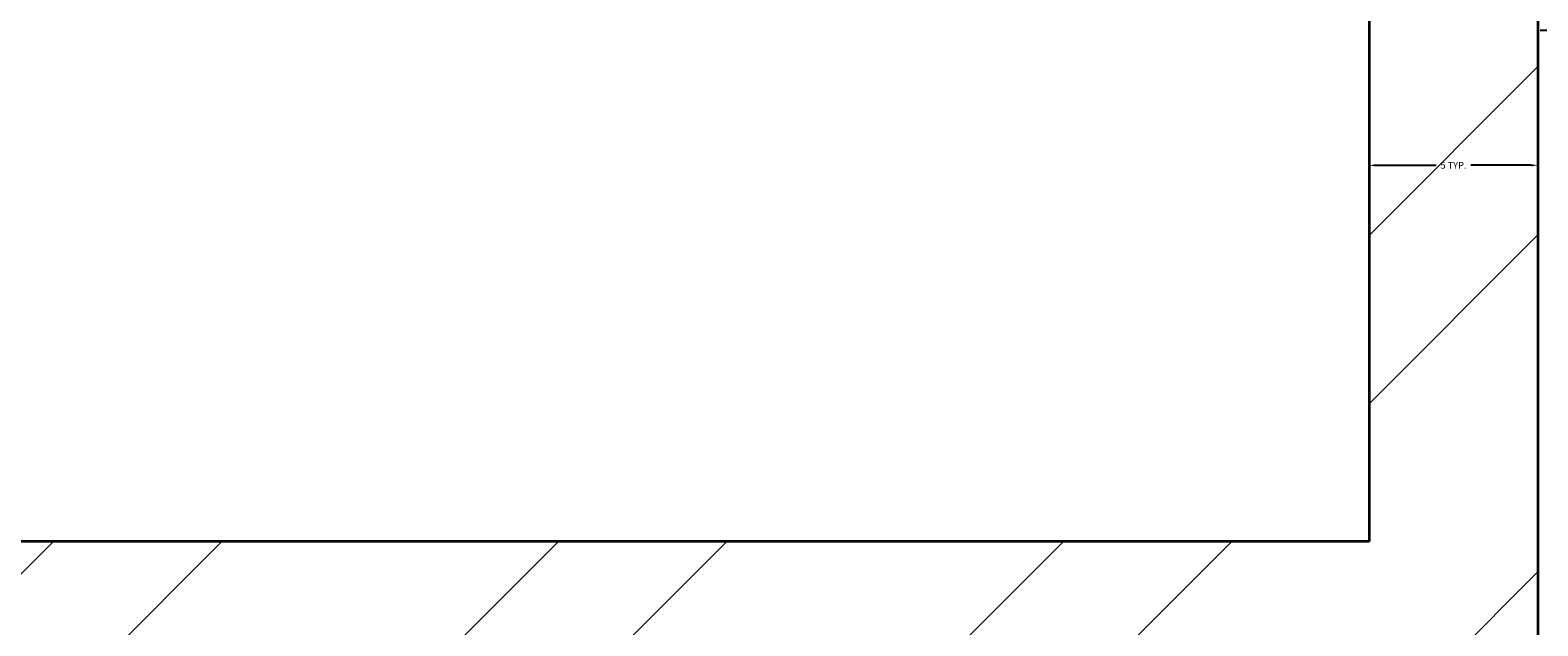
# Model space of a CAD drawing. Units: inches. Extents: x 1962 to 2771, y 1245 to 2660.
# Tile 17 of 114: x 2621 to 2661, y 1649 to 1665. Entities that reach past the tile are written whole.
import ezdxf

# ---------------------------------------------------------------- set-up
doc = ezdxf.new("R2010")
doc.units = ezdxf.units.IN
for name, color, linetype, lineweight in [('A-ANNO-DIMS', 2, 'Continuous', 18), ('A-WALL', 7, 'Continuous', 35), ('A-WALL-PATT', 252, 'Continuous', 13)]:
    doc.layers.add(name, color=color, linetype=linetype, lineweight=lineweight)
doc.styles.get("Standard").update_dxf_attribs({"font": 'arial.ttf'})
doc.dimstyles.get("Standard").update_dxf_attribs({"dimtxt": 0.18, "dimasz": 0.18, "dimexe": 0.18, "dimexo": 0.0625, "dimgap": 0.09, "dimtad": 0, "dimtih": 1, "dimtoh": 1, "dimdec": 4, "dimzin": 0, "dimdsep": 46, "dimtxsty": 'Standard', "dimcen": 0.09, "dimadec": 0, "dimazin": 0, "dimtfac": 1, "dimtdec": 4, "dimtofl": 0, "dimtmove": 0, "dimatfit": 3, "dimfxl": 1, "dimtolj": 1, "dimtzin": 0, "dimarcsym": 0})

# ---------------------------------------------------------------- blocks, each defined once
blk = doc.blocks.new('*D18')
at = {"layer": 'A-ANNO-DIMS', "color": 0, "lineweight": -2, "transparency": 16777216}
for p, q in [((2660.87, 1688.966), (2664.587, 1688.966)), ((2664.407, 1688.786), (2664.407, 1677.147)), ((2664.407, 1665.146), (2664.407, 1676.786)), ((2660.87, 1664.966), (2664.587, 1664.966))]:
    blk.add_line(p, q, dxfattribs=at)
at = {"layer": 'A-ANNO-DIMS', "color": 0, "transparency": 16777216}
for points in [[(2664.377, 1688.786), (2664.437, 1688.786), (2664.407, 1688.966)], [(2664.377, 1665.146), (2664.437, 1665.146), (2664.407, 1664.966)]]:
    blk.add_solid(points, dxfattribs=at)
at = {"layer": 'Defpoints', "color": 0, "transparency": 16777216}
for p in [(2660.807, 1688.966), (2664.407, 1688.966), (2660.807, 1664.966)]:
    blk.add_point(p, dxfattribs=at)
at = {"layer": 'A-ANNO-DIMS', "color": 0, "transparency": 16777216, "insert": (2664.407, 1676.966), "char_height": 0.18, "attachment_point": 5}
blk.add_mtext('\\A1;W1A 24 TYP.', dxfattribs=at)
blk = doc.blocks.new('*D19')
at = {"layer": 'A-ANNO-DIMS', "color": 0, "lineweight": -2, "transparency": 16777216}
for p, q in [((2656.307, 1664.904), (2656.307, 1661.186)), ((2660.807, 1664.904), (2660.807, 1661.186)), ((2656.487, 1661.366), (2658.099, 1661.366)), ((2660.627, 1661.366), (2659.016, 1661.366))]:
    blk.add_line(p, q, dxfattribs=at)
at = {"layer": 'A-ANNO-DIMS', "color": 0, "transparency": 16777216}
for points in [[(2656.487, 1661.396), (2656.487, 1661.336), (2656.307, 1661.366)], [(2660.627, 1661.396), (2660.627, 1661.336), (2660.807, 1661.366)]]:
    blk.add_solid(points, dxfattribs=at)
at = {"layer": 'Defpoints', "color": 0, "transparency": 16777216}
for p in [(2656.307, 1664.966), (2660.807, 1664.966), (2660.807, 1661.366)]:
    blk.add_point(p, dxfattribs=at)
at = {"layer": 'A-ANNO-DIMS', "color": 0, "transparency": 16777216, "insert": (2658.557, 1661.366), "char_height": 0.18, "attachment_point": 5}
blk.add_mtext('\\A1;5 TYP.', dxfattribs=at)

msp = doc.modelspace()

# ---------------------------------------------------------------- hatches: boundary and pattern name
at = {"layer": 'A-WALL-PATT'}
h = msp.add_hatch(dxfattribs=at)
h.set_pattern_fill('ANSI32', color=256)
h.paths.add_polyline_path([(2090.8074, 2467.3437), (2141.6481, 2467.3437), (2141.6481, 2469.5937), (2141.6481, 2471.8437), (2086.3074, 2471.8437), (2086.3074, 2422.5333), (2090.8074, 2422.5333)])
h.paths.add_polyline_path([(2282.7664, 2471.8437), (2204.8982, 2471.8437), (2204.8982, 2467.3437), (2234.8074, 2467.3437), (2234.8074, 2311.3437), (2228.7492, 2311.3437), (2228.7492, 2306.8437), (2234.8074, 2306.8437), (2331.9227, 2306.8437), (2331.9227, 2309.0937), (2331.9227, 2311.3437), (2239.3074, 2311.3437), (2239.3074, 2467.3437), (2282.7664, 2467.3437), (2282.7664, 2469.5937)])
h.paths.add_polyline_path([(2471.4531, 2519.8437), (2552.011, 2519.8437), (2564.3996, 2519.8437), (2564.3996, 2511.1389), (2568.8996, 2511.1389), (2568.8996, 2524.3437), (2466.9531, 2524.3437), (2466.9531, 2471.8437), (2450.0749, 2471.8437), (2446.4672, 2471.8437), (2446.4672, 2467.3437), (2450.0749, 2467.3437), (2475.9988, 2467.3437), (2475.9988, 2469.5937), (2475.9988, 2471.8437), (2471.4531, 2471.8437)])
h.paths.add_polyline_path([(2575.2231, 2469.5937), (2575.2231, 2471.8437), (2568.8996, 2471.8437), (2568.8996, 2487.1389), (2564.3996, 2487.1389), (2564.3996, 2471.8437), (2556.511, 2471.8437), (2499.2904, 2471.8437), (2499.2904, 2467.3437), (2507.8074, 2467.3437), (2507.8074, 2311.3437), (2414.863, 2311.3437), (2414.863, 2306.8437), (2512.3074, 2306.8437), (2517.0114, 2306.8437), (2517.0114, 2309.0937), (2517.0114, 2311.3437), (2512.3074, 2311.3437), (2512.3074, 2467.3437), (2575.2231, 2467.3437)])
h.paths.add_polyline_path([(2660.8074, 2471.8437), (2600.9602, 2471.8437), (2600.9602, 2467.3437), (2656.3074, 2467.3437), (2656.3074, 2432.5704), (2660.8074, 2432.5704)])
h.paths.add_polyline_path([(2660.8074, 2372.5704), (2656.3074, 2372.5704), (2656.3074, 2311.3437), (2600.276, 2311.3437), (2600.276, 2309.0937), (2600.276, 2306.8437), (2656.3074, 2306.8437), (2656.3074, 2296.2593), (2660.8074, 2296.2593)])
h.paths.add_polyline_path([(2572.3074, 2306.8437), (2577.1385, 2306.8437), (2577.1385, 2311.3437), (2551.082, 2311.3437), (2551.082, 2306.8437), (2567.8074, 2306.8437), (2567.8074, 2258.8437), (2540.0574, 2258.8437), (2540.0574, 2256.5937), (2540.0574, 2254.3437), (2567.8074, 2254.3437), (2656.3074, 2254.3437), (2656.3074, 2236.9085), (2660.8074, 2236.9085), (2660.8074, 2272.2593), (2656.3074, 2272.2593), (2656.3074, 2258.8437), (2572.3074, 2258.8437)])
h.paths.add_polyline_path([(2512.3074, 2254.3437), (2518.8716, 2254.3437), (2518.8716, 2256.5937), (2518.8716, 2258.8437), (2507.8074, 2258.8437), (2507.8074, 2177.8437), (2567.8074, 2177.8437), (2567.8074, 2172.9628), (2572.3074, 2172.9628), (2572.3074, 2177.8437), (2656.3074, 2177.8437), (2656.3074, 2166.4846), (2660.8074, 2166.4846), (2660.8074, 2200.9085), (2656.3074, 2200.9085), (2656.3074, 2182.3437), (2512.3074, 2182.3437)])
h.paths.add_polyline_path([(2656.3074, 2129.8437), (2572.3074, 2129.8437), (2572.3074, 2150.3044), (2570.0574, 2150.3044), (2567.8074, 2150.3044), (2567.8074, 2129.8437), (2507.8074, 2129.8437), (2507.8074, 2116.3027), (2510.0574, 2116.3027), (2512.3074, 2116.3027), (2512.3074, 2125.3437), (2567.8074, 2125.3437), (2572.3074, 2125.3437), (2656.3074, 2125.3437)])
h.paths.add_polyline_path([(2090.8074, 2362.5333), (2086.3074, 2362.5333), (2086.3074, 2298.6242), (2090.8074, 2298.6242), (2090.8074, 2306.8437), (2174.8074, 2306.8437), (2174.8074, 2286.4178), (2179.3074, 2286.4178), (2179.3074, 2306.8437), (2192.8641, 2306.8437), (2192.8641, 2309.0937), (2192.8641, 2311.3437), (2090.8074, 2311.3437)])
h.paths.add_polyline_path([(2209.156, 2258.8437), (2179.3074, 2258.8437), (2179.3074, 2263.2236), (2177.0574, 2263.2236), (2174.8074, 2263.2236), (2174.8074, 2258.8437), (2090.8074, 2258.8437), (2090.8074, 2274.6242), (2086.3074, 2274.6242), (2086.3074, 2238.2967), (2088.5574, 2238.2967), (2090.8074, 2238.2967), (2090.8074, 2254.3437), (2209.156, 2254.3437)])
h.paths.add_polyline_path([(2090.8074, 2177.8437), (2234.8074, 2177.8437), (2234.8074, 2173.1428), (2239.3074, 2173.1428), (2239.3074, 2258.8437), (2230.8442, 2258.8437), (2230.8442, 2256.5937), (2230.8442, 2254.3437), (2234.8074, 2254.3437), (2234.8074, 2182.3437), (2090.8074, 2182.3437), (2090.8074, 2202.2967), (2086.3074, 2202.2967), (2086.3074, 2140.0389), (2090.8074, 2140.0389)])
h.paths.add_polyline_path([(2090.8074, 2080.0389), (2086.3074, 2080.0389), (2086.3074, 2033.8437), (2090.8074, 2033.8437)], flags=17)
h.paths.add_polyline_path([(2244.9405, 2033.8437), (2239.3074, 2033.8437), (2239.3074, 2142.0665), (2237.2592, 2142.0665), (2234.8074, 2142.0665), (2234.8074, 2033.8437), (2090.8074, 2033.8437), (2076.5204, 2033.8437), (2072.0204, 2033.8437), (2072.0204, 2000.4493), (2076.5204, 2000.4493), (2076.5204, 2029.3437), (2090.8074, 2029.3437), (2244.9405, 2029.3437), (2244.9405, 2031.5937)])
h.paths.add_polyline_path([(2234.8074, 1933.3437), (2076.5204, 1933.3437), (2076.5204, 1952.4493), (2074.2704, 1952.4493), (2072.0204, 1952.4493), (2072.0204, 1933.3437), (2072.0204, 1928.8437), (2234.8074, 1928.8437)])
h.paths.add_polyline_path([(2090.8074, 1928.8437), (2086.3074, 1928.8437), (2086.3074, 1906.5013), (2090.8074, 1906.5013)])
h.paths.add_polyline_path([(2090.8074, 1846.5013), (2086.3074, 1846.5013), (2086.3074, 1769.9917), (2088.5574, 1769.9917), (2090.8074, 1769.9917), (2090.8074, 1780.3437), (2234.8074, 1780.3437), (2234.8074, 1708.3437), (2230.3764, 1708.3437), (2230.3764, 1703.8437), (2239.3074, 1703.8437), (2239.3074, 1792.6669), (2237.0574, 1792.6669), (2234.8074, 1792.6669), (2234.8074, 1784.8437), (2090.8074, 1784.8437)])
h.paths.add_polyline_path([(2239.3074, 1928.8437), (2244.9405, 1928.8437), (2244.9405, 1931.0937), (2244.9405, 1933.3437), (2234.8074, 1933.3437), (2234.8074, 1928.8437), (2234.8074, 1825.5949), (2239.3074, 1825.5949)])
h.paths.add_polyline_path([(2148.0425, 1649.0937), (2148.0425, 1651.3437), (2090.8074, 1651.3437), (2090.8074, 1646.8437), (2148.0425, 1646.8437)], flags=0)
h.paths.add_polyline_path([(2207.5601, 1708.3437), (2090.8074, 1708.3437), (2090.8074, 1703.8437), (2174.8074, 1703.8437), (2174.8074, 1651.3437), (2170.4457, 1651.3437), (2170.4457, 1646.8437), (2195.9924, 1646.8437), (2195.9924, 1649.0937), (2195.9924, 1651.3437), (2179.3074, 1651.3437), (2179.3074, 1703.8437), (2207.5601, 1703.8437), (2207.5601, 1706.0937)])
h.paths.add_polyline_path([(2090.8074, 1733.9917), (2086.3074, 1733.9917), (2086.3074, 1696.1032), (2088.5574, 1696.1032), (2090.8074, 1696.1032)])
h.paths.add_polyline_path([(2090.8074, 1672.1032), (2086.3074, 1672.1032), (2086.3074, 1600.3335), (2090.8074, 1600.3335)])
h.paths.add_polyline_path([(2090.8074, 1540.3335), (2086.3074, 1540.3335), (2086.3074, 1486.3437), (2139.6766, 1486.3437), (2139.6766, 1490.8437), (2090.8074, 1490.8437)])
h.paths.add_polyline_path([(2302.3876, 1490.8437), (2239.3074, 1490.8437), (2239.3074, 1646.8437), (2335.9994, 1646.8437), (2335.9994, 1651.3437), (2229.884, 1651.3437), (2229.884, 1646.8437), (2234.8074, 1646.8437), (2234.8074, 1490.8437), (2202.7103, 1490.8437), (2202.7103, 1488.5937), (2202.7103, 1486.3437), (2275.0699, 1486.3437), (2275.0699, 1475.772), (2279.5699, 1475.772), (2279.5699, 1486.3437), (2302.3876, 1486.3437)])
h.paths.add_polyline_path([(2279.5699, 1451.772), (2275.0699, 1451.772), (2275.0699, 1438.3437), (2174.8074, 1438.3437), (2174.8074, 1486.3437), (2179.7922, 1486.3437), (2179.7922, 1490.8437), (2163.3585, 1490.8437), (2163.3585, 1488.5937), (2163.3585, 1486.3437), (2170.3074, 1486.3437), (2170.3074, 1433.8437), (2279.5699, 1433.8437)])
h.paths.add_polyline_path([(2427.2363, 1490.8437), (2375.8074, 1490.8437), (2375.8074, 1646.8437), (2381.6401, 1646.8437), (2381.6401, 1651.3437), (2365.887, 1651.3437), (2365.887, 1649.0937), (2365.887, 1646.8437), (2371.3074, 1646.8437), (2371.3074, 1490.8437), (2327.5627, 1490.8437), (2327.5627, 1488.5937), (2327.5627, 1486.3437), (2371.3074, 1486.3437), (2371.3074, 1433.8437), (2375.8074, 1433.8437), (2375.8074, 1486.3437), (2427.2363, 1486.3437)])
h.paths.add_polyline_path([(2512.3074, 1646.8437), (2519.4351, 1646.8437), (2519.4351, 1649.0937), (2519.4351, 1651.3437), (2507.8074, 1651.3437), (2416.0063, 1651.3437), (2416.0063, 1649.0937), (2416.0063, 1646.8437), (2507.8074, 1646.8437), (2507.8074, 1490.8437), (2497.0532, 1490.8437), (2497.0532, 1488.5937), (2497.0532, 1486.3437), (2574.9344, 1486.3437), (2574.9344, 1476.0181), (2579.4344, 1476.0181), (2579.4344, 1486.3437), (2584.4872, 1486.3437), (2584.3074, 1490.8437), (2512.3074, 1490.8437)])
h.paths.add_polyline_path([(2470.5091, 1486.3437), (2473.9767, 1486.3437), (2473.9767, 1490.8437), (2449.6605, 1490.8437), (2449.6605, 1488.5937), (2449.6605, 1486.3437), (2466.0091, 1486.3437), (2466.0091, 1433.8437), (2470.5091, 1433.8437), (2579.4344, 1433.8437), (2579.4344, 1452.0181), (2574.9344, 1452.0181), (2574.9344, 1438.3437), (2554.5091, 1438.3437), (2470.5091, 1438.3437)])
h.paths.add_polyline_path([(2656.3074, 1490.8437), (2611.86, 1490.8437), (2611.86, 1486.3437), (2656.3074, 1486.3437)])
h.paths.add_polyline_path([(2660.8074, 1532.7007), (2658.5574, 1532.7007), (2656.3074, 1532.7007), (2656.3074, 1486.3437), (2660.8074, 1486.3437)])
h.paths.add_polyline_path([(2660.8074, 1664.9663), (2656.3074, 1664.9663), (2656.3074, 1651.3437), (2602.2313, 1651.3437), (2602.2313, 1646.8437), (2656.3074, 1646.8437), (2656.3074, 1592.7007), (2660.8074, 1592.7007)])
h.paths.add_polyline_path([(2660.8074, 1724.5221), (2656.3074, 1724.5221), (2656.3074, 1703.8437), (2542.4725, 1703.8437), (2542.4725, 1699.3437), (2567.8074, 1699.3437), (2567.8074, 1651.3437), (2552.7766, 1651.3437), (2552.7766, 1649.0937), (2552.7766, 1646.8437), (2577.2878, 1646.8437), (2577.2878, 1649.0937), (2577.2878, 1651.3437), (2572.3074, 1651.3437), (2572.3074, 1699.3437), (2656.3074, 1699.3437), (2656.3074, 1688.9663), (2660.8074, 1688.9663)])
h.paths.add_polyline_path([(2660.8074, 1880.6524), (2656.3074, 1880.6524), (2656.3074, 1832.8437), (2512.3074, 1832.8437), (2512.3074, 1837.8959), (2507.8074, 1837.8959), (2507.8074, 1828.3437), (2567.8074, 1828.3437), (2567.8074, 1804.3437), (2572.3074, 1804.3437), (2572.3074, 1828.3437), (2656.3074, 1828.3437), (2656.3074, 1818.6778), (2660.8074, 1818.6778)])
h.paths.add_polyline_path([(2660.8074, 1794.6778), (2656.3074, 1794.6778), (2656.3074, 1780.3437), (2572.3074, 1780.3437), (2572.3074, 1783.0303), (2570.0574, 1783.0303), (2567.8074, 1783.0303), (2567.8074, 1780.3437), (2507.8074, 1780.3437), (2507.8074, 1699.3437), (2517.8858, 1699.3437), (2517.8858, 1701.5937), (2517.8858, 1703.8437), (2512.3074, 1703.8437), (2512.3074, 1775.8437), (2656.3074, 1775.8437), (2656.3074, 1760.5221), (2660.8074, 1760.5221)])
h.paths.add_polyline_path([(2660.8074, 1981.3437), (2660.8074, 2020.2808), (2658.5574, 2020.2808), (2656.3074, 2020.2808), (2656.3074, 1981.3437), (2512.3074, 1981.3437), (2512.3074, 2086.6996), (2507.8074, 2086.6996), (2507.8074, 1981.3437), (2375.8074, 1981.3437), (2375.8074, 1986.8505), (2373.5574, 1986.8505), (2371.3074, 1986.8505), (2371.3074, 1973.2607), (2375.8074, 1973.2607), (2375.8074, 1976.8437), (2507.8074, 1976.8437), (2507.8074, 1865.4281), (2510.0574, 1865.4281), (2512.3074, 1865.4281), (2512.3074, 1976.8437), (2660.8074, 1976.8437)])
h.paths.add_polyline_path([(2375.8074, 1940.297), (2373.5574, 1940.297), (2371.3074, 1940.297), (2371.3074, 1933.3437), (2278.4434, 1933.3437), (2278.4434, 1928.8437), (2371.3074, 1928.8437), (2371.3074, 1651.3437), (2375.8074, 1651.3437)])
h.paths.add_polyline_path([(2660.8074, 1976.8437), (2656.3074, 1976.8437), (2656.3074, 1940.6524), (2660.8074, 1940.6524)], flags=17)
h.paths.add_polyline_path([(2660.8074, 2142.4846), (2656.3074, 2142.4846), (2656.3074, 2080.2808), (2660.8074, 2080.2808)])
h.paths.add_polyline_path([(2381.4189, 2311.3437), (2375.8074, 2311.3437), (2375.8074, 2467.3437), (2424.7242, 2467.3437), (2424.7242, 2469.5937), (2424.7242, 2471.8437), (2375.8074, 2471.8437), (2375.8074, 2524.3437), (2371.3074, 2524.3437), (2371.3074, 2471.8437), (2307.2097, 2471.8437), (2307.2097, 2467.3437), (2371.3074, 2467.3437), (2371.3074, 2311.3437), (2366.8901, 2311.3437), (2366.8901, 2306.8437), (2371.3074, 2306.8437), (2371.3074, 2033.8437), (2279.6589, 2033.8437), (2279.6589, 2029.3437), (2371.3074, 2029.3437), (2371.3074, 2014.2598), (2375.8074, 2014.2598), (2375.8074, 2306.8437), (2381.4189, 2306.8437)])
h.paths.add_polyline_path([(2263.3074, 2524.3437), (2170.3074, 2524.3437), (2170.3074, 2519.8437), (2170.3074, 2471.8437), (2165.0312, 2471.8437), (2165.0312, 2467.3437), (2179.6721, 2467.3437), (2179.6721, 2469.5161), (2179.6721, 2471.8437), (2174.8074, 2471.8437), (2174.8074, 2519.8437), (2258.8074, 2519.8437), (2258.8074, 2511.6436), (2263.3074, 2511.6436)])
h.paths.add_polyline_path([(2245.0232, 1361.4123), (2492.9468, 1361.4123), (2492.9468, 1398.505), (2245.0232, 1398.505)], flags=9)
h.paths.add_polyline_path([(2388.1434, 2086.6936), (2425.0704, 2086.6936), (2425.0704, 2105.3509), (2388.1434, 2105.3509)], flags=9)
h.paths.add_polyline_path([(2404.922, 2242.6744), (2445.7337, 2242.6744), (2445.7337, 2261.3318), (2404.922, 2261.3318)], flags=9)
h.paths.add_polyline_path([(2269.4107, 2156.7935), (2306.3378, 2156.7935), (2306.3378, 2175.4508), (2269.4107, 2175.4508)], flags=9)
h.paths.add_polyline_path([(2269.3277, 2233.4343), (2306.2547, 2233.4343), (2306.2547, 2252.0917), (2269.3277, 2252.0917)], flags=9)
h.paths.add_polyline_path([(2431.6052, 2320.6922), (2470.4456, 2320.6922), (2470.4456, 2339.3495), (2431.6052, 2339.3495)], flags=25)
h.paths.add_polyline_path([(2249.6902, 2315.7608), (2288.5306, 2315.7608), (2288.5306, 2334.4182), (2249.6902, 2334.4182)], flags=25)
h.paths.add_polyline_path([(2096.9301, 2314.3181), (2135.7704, 2314.3181), (2135.7704, 2332.9755), (2096.9301, 2332.9755)], flags=25)
h.paths.add_polyline_path([(2134.3475, 2285.7089), (2161.4655, 2285.7089), (2161.4655, 2304.3662), (2134.3475, 2304.3662)], flags=9)
h.paths.add_polyline_path([(2126.5155, 2209.4076), (2159.9227, 2209.4076), (2159.9227, 2228.065), (2126.5155, 2228.065)], flags=25)
h.paths.add_polyline_path([(2110.5753, 2141.5299), (2149.4157, 2141.5299), (2149.4157, 2160.1872), (2110.5753, 2160.1872)], flags=25)
h.paths.add_polyline_path([(2249.8618, 1968.3317), (2286.3966, 1968.3317), (2286.3966, 1986.989), (2249.8618, 1986.989)], flags=9)
h.paths.add_polyline_path([(2395.9507, 1777.0051), (2436.7624, 1777.0051), (2436.7624, 1795.6625), (2395.9507, 1795.6625)], flags=9)
h.paths.add_polyline_path([(2398.5259, 1888.5651), (2435.0062, 1888.5651), (2435.0062, 1907.2224), (2398.5259, 1907.2224)], flags=25)
h.paths.add_polyline_path([(2259.3506, 1728.3559), (2296.2776, 1728.3559), (2296.2776, 1747.0132), (2259.3506, 1747.0132)], flags=9)
h.paths.add_polyline_path([(2271.3698, 1845.268), (2308.2968, 1845.268), (2308.2968, 1863.9253), (2271.3698, 1863.9253)], flags=9)
h.paths.add_polyline_path([(2120.9355, 1786.3027), (2159.7759, 1786.3027), (2159.7759, 1804.9601), (2120.9355, 1804.9601)], flags=25)
h.paths.add_polyline_path([(2121.3164, 1732.1043), (2154.7236, 1732.1043), (2154.7236, 1750.7616), (2121.3164, 1750.7616)], flags=25)
h.paths.add_polyline_path([(2118.3706, 1678.8997), (2147.5282, 1678.8997), (2147.5282, 1697.557), (2118.3706, 1697.557)], flags=25)
h.paths.add_polyline_path([(2385.9227, 1493.557), (2424.763, 1493.557), (2424.763, 1512.2143), (2385.9227, 1512.2143)], flags=25)
h.paths.add_polyline_path([(2248.7058, 1500.0256), (2287.5462, 1500.0256), (2287.5462, 1518.6829), (2248.7058, 1518.6829)], flags=25)
h.paths.add_polyline_path([(2104.1669, 1617.3771), (2143.0073, 1617.3771), (2143.0073, 1636.0344), (2104.1669, 1636.0344)], flags=9)
h.paths.add_polyline_path([(2096.0714, 1447.8824), (2137.3845, 1447.8824), (2137.3845, 1458.1859), (2096.0714, 1458.1859)], flags=9)
h.paths.add_polyline_path([(2180.6114, 1440.325), (2209.7689, 1440.325), (2209.7689, 1458.9823), (2180.6114, 1458.9823)], flags=25)
h.paths.add_polyline_path([(2316.1698, 1447.9637), (2357.4829, 1447.9637), (2357.4829, 1458.2673), (2316.1698, 1458.2673)], flags=9)
h.paths.add_polyline_path([(2397.6187, 1447.9637), (2438.9318, 1447.9637), (2438.9318, 1458.2673), (2397.6187, 1458.2673)], flags=9)
h.paths.add_polyline_path([(2473.0778, 1439.5953), (2502.2354, 1439.5953), (2502.2354, 1458.2527), (2473.0778, 1458.2527)], flags=25)
h.paths.add_polyline_path([(2589.7027, 1447.8819), (2631.0158, 1447.8819), (2631.0158, 1458.1855), (2589.7027, 1458.1855)], flags=9)
h.paths.add_polyline_path([(2522.4009, 1497.5285), (2561.2413, 1497.5285), (2561.2413, 1516.1859), (2522.4009, 1516.1859)], flags=25)
h.paths.add_polyline_path([(2579.6565, 1671.3482), (2608.8141, 1671.3482), (2608.8141, 1690.0056), (2579.6565, 1690.0056)], flags=25)
h.paths.add_polyline_path([(2544.7038, 1725.5064), (2578.1111, 1725.5064), (2578.1111, 1744.1637), (2544.7038, 1744.1637)], flags=25)
h.paths.add_polyline_path([(2578.1191, 1807.472), (2607.2766, 1807.472), (2607.2766, 1826.1293), (2578.1191, 1826.1293)], flags=25)
h.paths.add_polyline_path([(2595.0614, 1835.1839), (2633.9018, 1835.1839), (2633.9018, 1853.8413), (2595.0614, 1853.8413)], flags=25)
h.paths.add_polyline_path([(2567.0097, 2097.7035), (2605.8501, 2097.7035), (2605.8501, 2116.3609), (2567.0097, 2116.3609)], flags=9)
h.paths.add_polyline_path([(2586.644, 2134.6454), (2615.8015, 2134.6454), (2615.8015, 2153.3027), (2586.644, 2153.3027)], flags=9)
h.paths.add_polyline_path([(2544.6185, 2212.6783), (2578.0258, 2212.6783), (2578.0258, 2231.3356), (2544.6185, 2231.3356)], flags=25)
h.paths.add_polyline_path([(2577.0273, 2256.9023), (2606.1849, 2256.9023), (2606.1849, 2275.5597), (2577.0273, 2275.5597)], flags=24)
h.paths.add_polyline_path([(2605.2683, 2315.2821), (2644.1087, 2315.2821), (2644.1087, 2333.9395), (2605.2683, 2333.9395)], flags=25)
h.paths.add_polyline_path([(2583.1244, 2496.1815), (2624.4375, 2496.1815), (2624.4375, 2506.4851), (2583.1244, 2506.4851)], flags=9)
h.paths.add_polyline_path([(2474.761, 2497.0823), (2503.9185, 2497.0823), (2503.9185, 2515.7397), (2474.761, 2515.7397)], flags=25)
h.paths.add_polyline_path([(2387.5787, 2494.2563), (2428.902, 2494.2563), (2428.902, 2504.5598), (2387.5787, 2504.5598)], flags=9)
h.paths.add_polyline_path([(2300.1657, 2500.1564), (2341.4788, 2500.1564), (2341.4788, 2510.46), (2300.1657, 2510.46)], flags=25)
h.paths.add_polyline_path([(2176.8589, 2497.5843), (2206.0165, 2497.5843), (2206.0165, 2516.2416), (2176.8589, 2516.2416)], flags=25)
h.paths.add_polyline_path([(2097.4668, 2494.9762), (2138.7799, 2494.9762), (2138.7799, 2505.2798), (2097.4668, 2505.2798)], flags=9)

# ---------------------------------------------------------------- linework, layer by layer
at = {"layer": 'A-WALL'}
for p, q in [((2660.8074, 1976.8437), (2660.8074, 1486.3437)), ((2656.3074, 1699.3437), (2656.3074, 1651.3437)), ((2656.3074, 1651.3437), (2600.4171, 1651.3437))]:
    msp.add_line(p, q, dxfattribs=at)

# ---------------------------------------------------------------- dimensions: what is measured, and where the dimension line sits
at = {"layer": 'A-ANNO-DIMS'}
dim = msp.add_linear_dim(base=(2664.4074, 1688.9663), p1=(2660.8074, 1664.9663), p2=(2660.8074, 1688.9663), angle=90, text='W1A <> TYP.', dimstyle='Standard', override={"dimdec": 0, "dimlfac": 1, "dimrnd": 0, "dimzin": 0, "dimdsep": 46, "dimlunit": 2}, dxfattribs=at)
dim.commit()
dim.dimension.update_dxf_attribs({"geometry": '*D18', "text_midpoint": (2664.4074, 1676.9663)})
dim = msp.add_linear_dim(base=(2660.8073805882, 1661.3663245259), p1=(2656.3073805882, 1664.9663245259), p2=(2660.8073805882, 1664.9663245259), text='<> TYP.', dimstyle='Standard', override={"dimdec": 0, "dimlfac": 1, "dimrnd": 0, "dimzin": 0, "dimdsep": 46, "dimlunit": 2}, dxfattribs=at)
dim.commit()
dim.dimension.update_dxf_attribs({"geometry": '*D19', "text_midpoint": (2658.5573805882, 1661.3663245259)})

doc.saveas('drawing.dxf')
